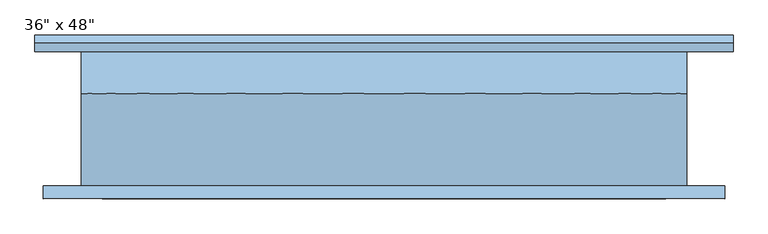
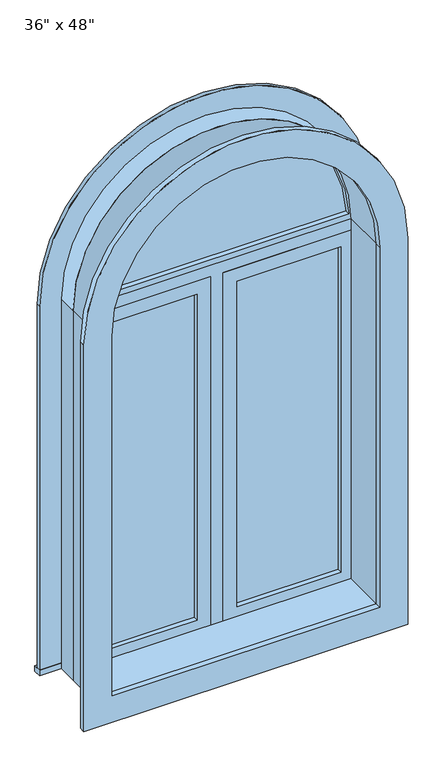
"""IFC4 building model written with IfcOpenShell, lengths in millimetres: window geometry."""

from ifc_helpers import new_model, si_unit, point, frame, frame_2d, origin, place, context, project, spatial, polyline, circle_curve, trimmed, segment, composite_curve, outline, extrude, source, transform, mapped, element, save


def window_cf4adaea(model_context):
    return source(origin(), model_context, "Body", "SweptSolid", [
        extrude(outline(composite_curve([segment(polyline([(2152.65, -506.3478419), (857.25, -506.3478419), (857.25, 522.3521581), (2152.65, 522.3521581)]), True, "CONTINUOUS"), segment(trimmed(circle_curve(frame_2d((2152.65, 8.0021581)), 514.35), [point((2152.65, 522.3521581))], [point((2152.65, -506.3478419))], False, "CARTESIAN"), True, "CONTINUOUS")], self_intersect=False), holes=[composite_curve([segment(trimmed(circle_curve(frame_2d((2152.65, 8.0021581)), 425.45), [point((2152.65, -417.4478419))], [point((2152.65, 433.4521581))], True, "CARTESIAN"), True, "CONTINUOUS"), segment(polyline([(2152.65, 433.4521581), (946.15, 433.4521581), (946.15, -417.4478419), (2152.65, -417.4478419)]), True, "CONTINUOUS")], self_intersect=False)]), frame((0.0, -120.65, 0.0), z_axis=(0.0, 1.0, 0.0), x_axis=(0.0, 0.0, 1.0)), (0.0, 0.0, 1.0), 19.05),
        extrude(outline(composite_curve([segment(trimmed(circle_curve(frame_2d((2152.65, 8.0021581)), 419.2154707), [point((2171.6999995, 426.7845699))], [point((2171.6999995, -410.7802537))], False, "CARTESIAN"), True, "CONTINUOUS"), segment(polyline([(2171.6999995, -410.7802537), (2171.6999995, 426.7845699)]), True, "CONTINUOUS")], self_intersect=False)), frame((0.0, 53.975, 0.0), z_axis=(0.0, 1.0, 0.0), x_axis=(0.0, 0.0, 1.0)), (0.0, 0.0, 1.0), 12.7),
        extrude(outline(composite_curve([segment(trimmed(circle_curve(frame_2d((2152.65, 8.0021581)), 438.15), [point((2152.65, 446.1521581))], [point((2152.65, -430.1478419))], False, "CARTESIAN"), True, "CONTINUOUS"), segment(polyline([(2152.65, -430.1478419), (2152.65, 446.1521581)]), True, "CONTINUOUS")], self_intersect=False), holes=[composite_curve([segment(polyline([(2171.6999995, 426.7845698), (2171.6999995, -410.7802537)]), True, "CONTINUOUS"), segment(trimmed(circle_curve(frame_2d((2152.65, 8.0021581)), 419.2154707), [point((2171.6999995, -410.7802537))], [point((2171.6999995, 426.7845698))], True, "CARTESIAN"), True, "CONTINUOUS")], self_intersect=False)]), frame((0.0, 38.1, 0.0), z_axis=(0.0, 1.0, 0.0), x_axis=(0.0, 0.0, 1.0)), (0.0, 0.0, 1.0), 44.45),
        extrude(outline(composite_curve([segment(polyline([(914.4, -449.1978419), (914.4, 465.2021581), (2152.65, 465.2021581)]), True, "CONTINUOUS"), segment(trimmed(circle_curve(frame_2d((2152.65, 8.0021581)), 457.2), [point((2152.65, 465.2021581))], [point((2152.65, -449.1978419))], False, "CARTESIAN"), True, "CONTINUOUS"), segment(polyline([(2152.65, -449.1978419), (914.4, -449.1978419)]), True, "CONTINUOUS")], self_intersect=False), holes=[composite_curve([segment(polyline([(933.45, -430.1478419), (2152.65, -430.1478419)]), True, "CONTINUOUS"), segment(trimmed(circle_curve(frame_2d((2152.65, 8.0021581)), 438.15), [point((2152.65, -430.1478419))], [point((2152.65, 446.1521581))], True, "CARTESIAN"), True, "CONTINUOUS"), segment(polyline([(2152.65, 446.1521581), (933.45, 446.1521581), (933.45, -430.1478419)]), True, "CONTINUOUS")], self_intersect=False)]), frame((0.0, 38.1, 0.0), z_axis=(0.0, 1.0, 0.0), x_axis=(0.0, 0.0, 1.0)), (0.0, 0.0, 1.0), 63.5),
        extrude(outline(polyline([(71.5021581, 66.675), (401.7021581, 66.675), (401.7021581, 53.975), (71.5021581, 53.975), (71.5021581, 66.675)])), frame((0.0, 0.0, 977.9), z_axis=(0.0, 0.0, 1.0), x_axis=(1.0, 0.0, 0.0)), (0.0, 0.0, 1.0), 1092.2),
        extrude(outline(polyline([(2114.55, 27.0521581), (933.45, 27.0521581), (933.45, 446.1521581), (2114.55, 446.1521581), (2114.55, 27.0521581)]), holes=[polyline([(2070.1, 71.5021581), (2070.1, 401.7021581), (977.9, 401.7021581), (977.9, 71.5021581), (2070.1, 71.5021581)])]), frame((0.0, 38.1, 0.0), z_axis=(0.0, 1.0, 0.0), x_axis=(0.0, 0.0, 1.0)), (0.0, 0.0, 1.0), 44.45),
        extrude(outline(polyline([(933.45, -11.0478419), (933.45, 27.0521581), (2114.55, 27.0521581), (2114.55, 446.1521581), (2152.65, 446.1521581), (2152.65, -430.1478419), (2114.55, -430.1478419), (2114.55, -11.0478419), (933.45, -11.0478419)])), frame((0.0, 38.1, 0.0), z_axis=(0.0, 1.0, 0.0), x_axis=(0.0, 0.0, 1.0)), (0.0, 0.0, 1.0), 63.5),
        extrude(outline(polyline([(-519.0478419, 127.0), (535.0521581, 127.0), (535.0521581, 101.6), (-519.0478419, 101.6), (-519.0478419, 127.0)])), frame((0.0, 0.0, 914.4), z_axis=(0.0, 0.0, 1.0), x_axis=(1.0, 0.0, 0.0)), (0.0, 0.0, 1.0), 19.05),
        extrude(outline(composite_curve([segment(polyline([(933.45, 446.1521581), (933.45, 535.0521581), (2152.65, 535.0521581)]), True, "CONTINUOUS"), segment(trimmed(circle_curve(frame_2d((2152.65, 8.0021581)), 527.05), [point((2152.65, 535.0521581))], [point((2152.65, -519.0478419))], False, "CARTESIAN"), True, "CONTINUOUS"), segment(polyline([(2152.65, -519.0478419), (933.45, -519.0478419), (933.45, -430.1478419), (2152.65, -430.1478419)]), True, "CONTINUOUS"), segment(trimmed(circle_curve(frame_2d((2152.65, 8.0021581)), 438.15), [point((2152.65, -430.1478419))], [point((2152.65, 446.1521581))], True, "CARTESIAN"), True, "CONTINUOUS"), segment(polyline([(2152.65, 446.1521581), (933.45, 446.1521581)]), True, "CONTINUOUS")], self_intersect=False)), frame((0.0, 101.6, 0.0), z_axis=(0.0, 1.0, 0.0), x_axis=(0.0, 0.0, 1.0)), (0.0, 0.0, 1.0), 12.7),
        extrude(outline(polyline([(-55.4978419, 53.975), (-385.6978419, 53.975), (-385.6978419, 66.675), (-55.4978419, 66.675), (-55.4978419, 53.975)])), frame((0.0, 0.0, 977.9), z_axis=(0.0, 0.0, 1.0), x_axis=(1.0, 0.0, 0.0)), (0.0, 0.0, 1.0), 1092.2),
        extrude(outline(polyline([(2114.55, -430.1478419), (933.45, -430.1478419), (933.45, -11.0478419), (2114.55, -11.0478419), (2114.55, -430.1478419)]), holes=[polyline([(2070.1, -385.6978419), (2070.1, -55.4978419), (977.9, -55.4978419), (977.9, -385.6978419), (2070.1, -385.6978419)])]), frame((0.0, 38.1, 0.0), z_axis=(0.0, 1.0, 0.0), x_axis=(0.0, 0.0, 1.0)), (0.0, 0.0, 1.0), 44.45),
        extrude(outline(composite_curve([segment(polyline([(914.4, 465.2021581), (2152.65, 465.2021581)]), True, "CONTINUOUS"), segment(trimmed(circle_curve(frame_2d((2152.65, 8.0021581)), 457.2), [point((2152.65, 465.2021581))], [point((2152.65, -449.1978419))], False, "CARTESIAN"), True, "CONTINUOUS"), segment(polyline([(2152.65, -449.1978419), (914.4, -449.1978419), (914.4, 465.2021581)]), True, "CONTINUOUS")], self_intersect=False), holes=[composite_curve([segment(polyline([(946.15, 433.4521581), (946.15, -417.4478419), (2152.65, -417.4478419)]), True, "CONTINUOUS"), segment(trimmed(circle_curve(frame_2d((2152.65, 8.0021581)), 425.45), [point((2152.65, -417.4478419))], [point((2152.65, 433.4521581))], True, "CARTESIAN"), True, "CONTINUOUS"), segment(polyline([(2152.65, 433.4521581), (946.15, 433.4521581)]), True, "CONTINUOUS")], self_intersect=False)]), frame((0.0, -101.6, 0.0), z_axis=(0.0, 1.0, 0.0), x_axis=(0.0, 0.0, 1.0)), (0.0, 0.0, 1.0), 139.7),
    ])


if __name__ == "__main__":
    model = new_model("IFC4")
    model_context = context("Model", 3, world=origin())
    ifc_project = project(units=[si_unit("LENGTHUNIT", "METRE", prefix="MILLI")], contexts=[model_context])
    site = spatial("IfcSite", under=ifc_project)
    building = spatial("IfcBuilding", under=site)
    placement = place(None, origin())
    window_shape = window_cf4adaea(model_context)
    element("IfcWindow", 1, ObjectType="36\" x 48\"", at=placement, inside=building, context=model_context, shape_type="MappedRepresentation", body=[
        mapped(window_shape, transform((0.0, 0.0, 0.0), x_axis=(1.0, 0.0, 0.0), y_axis=(0.0, 1.0, 0.0), z_axis=(0.0, 0.0, 1.0))),
    ])
    save(model, "model.ifc")

# Revit data of these elements
# Type "36\" x 48\""
#   Type Mark = "38"
#   Construction Type Id = "SGL"
#   Assembly Code = "B2020100"
#   Analytic Construction = "Large single-glazed windows"
#   Visual Light Transmittance = 0.9
#   Solar Heat Gain Coefficient = 0.86
#   Heat Transfer Coefficient (U) = 0.979472 BTU/(h·ft²·°F)
#   Height = 4' - 0"
#   Default Sill Height = 3' - 0"
#   Trim Projection - Ext. = 0' - 0 1/2"
#   Trim Projection - Int. = 0' - 0 3/4"
#   Trim Width - Exterior = 0' - 3 1/2"
#   Trim Width - Interior = 0' - 3 1/2"
#   Width = 3' - 0"
#   Window Inset = 0' - 0 3/4"
#   Define Thermal Properties by = 1
#   Glass Pane Material = Glass
#   Sash Material = Sash
#   Trim Exterior Material = Trim
#   Trim Interior Material = Trim
#   Wall Closure = (empty or 0)
# Element 1 (IfcWindow, "36\" x 48\"")
#   Materials on its faces: "Sash", "Trim", "Glass"
# Materials
#   "Glass": class "Glass", colour RGB 0 128 192, transparency 0.75, Description = "Soda Lime Glass", Cost = 0
#   "Sash": class "Wood", colour RGB 224 178 126, transparency 0
#   "Trim": class "Wood", colour RGB 224 178 126, transparency 0
